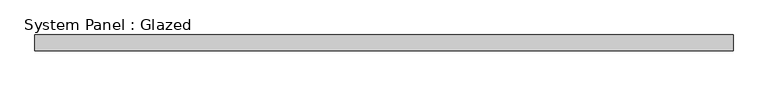
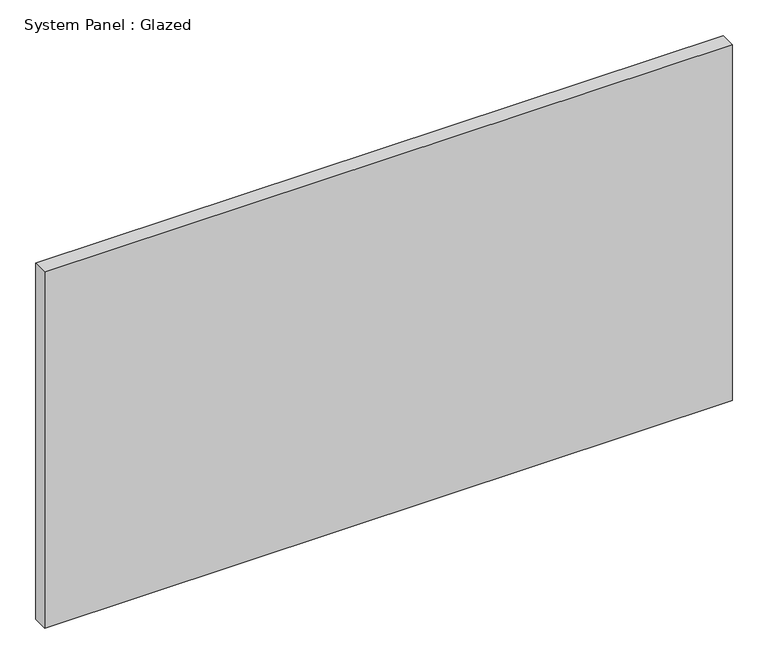
"""IFC4 building model written with IfcOpenShell, lengths in millimetres: plate geometry, System Panel : Glazed."""

from ifc_helpers import new_model, si_unit, origin, origin_with_axes, place, context, project, spatial, polyline, outline, extrude, source, transform, mapped, element, save


def system_panel_glazed_2ebb08bf(model_context):
    return source(origin(), model_context, "Body", "SweptSolid", [
        extrude(outline(polyline([(556.3186962, 24.5), (-556.3186962, 24.5), (-556.3186962, 49.5), (556.3186962, 49.5), (556.3186962, 24.5)])), origin_with_axes(), (0.0, 0.0, 1.0), 609.6),
    ])


if __name__ == "__main__":
    model = new_model("IFC4")
    model_context = context("Model", 3, world=origin())
    ifc_project = project(units=[si_unit("LENGTHUNIT", "METRE", prefix="MILLI")], contexts=[model_context])
    site = spatial("IfcSite", under=ifc_project)
    building = spatial("IfcBuilding", under=site)
    placement = place(None, origin())
    system_panel_glazed_shape = system_panel_glazed_2ebb08bf(model_context)
    element("IfcPlate", 1, ObjectType="System Panel : Glazed", at=placement, inside=building, context=model_context, shape_type="MappedRepresentation", body=[
        mapped(system_panel_glazed_shape, transform((0.0, 0.0, 0.0), x_axis=(1.0, 0.0, 0.0), y_axis=(0.0, 1.0, 0.0), z_axis=(0.0, 0.0, 1.0))),
    ])
    save(model, "model.ifc")

# Revit data of these elements
# Type "System Panel : Glazed"
#   Keynote = "H11"
#   Construction Type Id = "GSP4R"
#   Analytic Construction = "1/8 in Pilkington single glazing"
#   Visual Light Transmittance = 0.9
#   Solar Heat Gain Coefficient = 0.86
#   Heat Transfer Coefficient (U) = 6.7069 W/(m²·K)
#   Define Thermal Properties by = 1
# Element 1 (IfcPlate, "System Panel : Glazed")
#   Materials on its faces: "Glass"
# Materials
#   "Glass": class "Glass", colour RGB 0 128 192, transparency 0.9, Description = "Soda Lime Glass", Cost = 0
